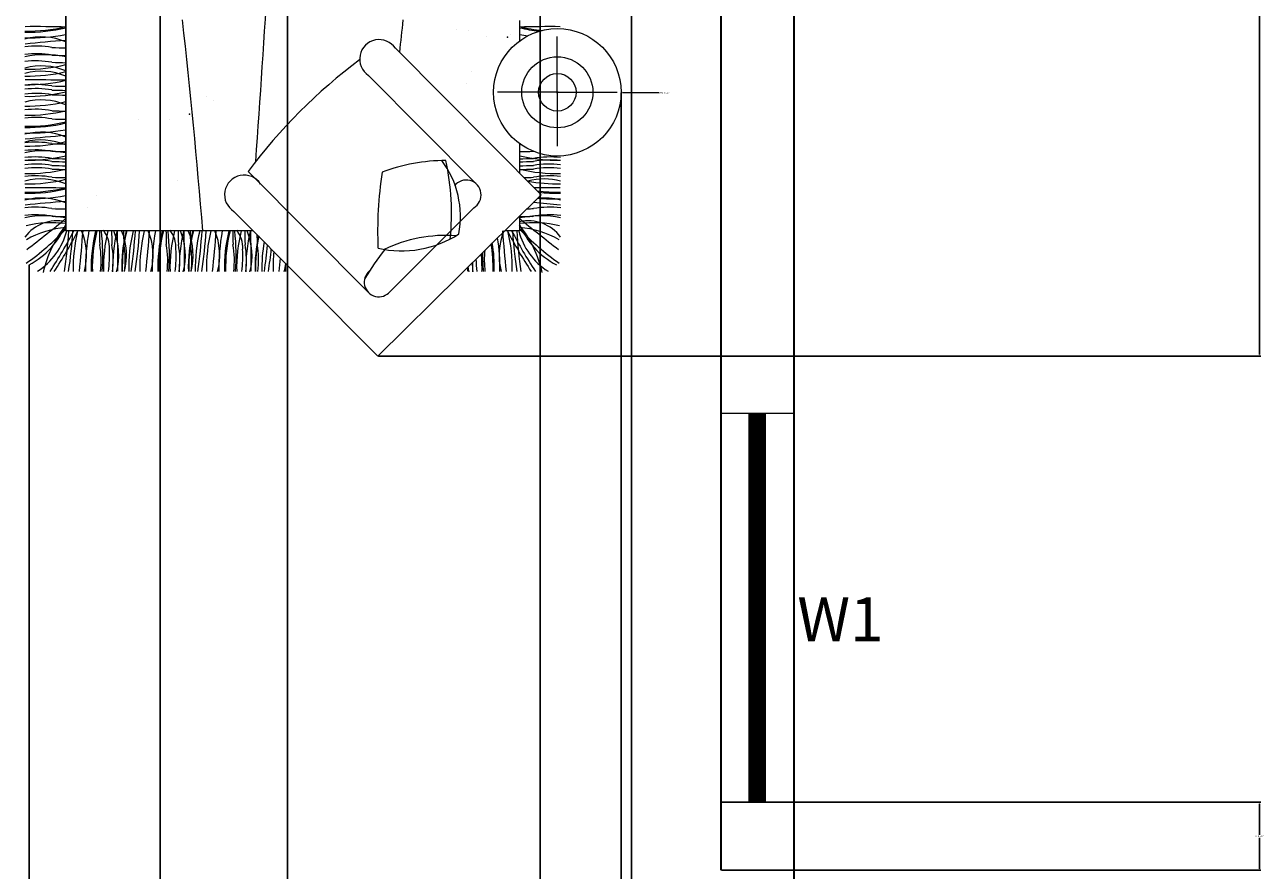
# Model space of a CAD drawing. Units: inches. Extents: x 318 to 927, y -1130 to 13.
# Tile 10 of 17: x 774 to 927, y -692 to -587. Entities that reach past the tile are written whole.
import ezdxf

# ---------------------------------------------------------------- set-up
doc = ezdxf.new("R2010")
doc.units = ezdxf.units.IN
doc.header["$MEASUREMENT"] = 0
for name, color, linetype, lineweight in [('A-ANNO-DIMS', 1, 'Continuous', 18), ('A-ANNO-IDEN', 1, 'Continuous', 13), ('A-FURN-RUGS', 50, 'Continuous', 9), ('A-GLAZ-PATT', 5, 'Continuous', 9), ('wall', 1, 'Continuous', 35), ('win', 5, 'Continuous', 18)]:
    doc.layers.add(name, color=color, linetype=linetype, lineweight=lineweight)
doc.layers.add('furniture', color=50, linetype='Continuous', lineweight=13, transparency=0.8)
doc.styles.get("Standard").update_dxf_attribs({"font": 'arial.ttf'})
doc.dimstyles.get("Standard").update_dxf_attribs({"dimtxt": 0.18, "dimasz": 0.18, "dimexe": 0.18, "dimexo": 0.0625, "dimgap": 0.09, "dimtad": 0, "dimtih": 1, "dimtoh": 1, "dimdec": 1, "dimzin": 0, "dimdsep": 46, "dimlunit": 4, "dimtxsty": 'Standard', "dimcen": 0.09, "dimadec": 0, "dimazin": 0, "dimtfac": 1, "dimtdec": 1, "dimtofl": 0, "dimtmove": 0, "dimatfit": 3, "dimfxl": 1, "dimtolj": 1, "dimtzin": 0, "dimarcsym": 0})

# ---------------------------------------------------------------- blocks, each defined once
blk = doc.blocks.new('WIN-48IN')
for p, q in [((0, 48), (9, 48)), ((3.5, 48), (3.5, 0)), ((5.5, 48), (5.5, 0)), ((0, 0), (9, 0))]:
    blk.add_line(p, q)
blk = doc.blocks.new('*D38')
at = {"layer": 'A-ANNO-DIMS', "color": 0, "lineweight": -2, "transparency": 16777216}
for p, q in [((817.59, -493.51), (926.57, -493.51)), ((926.39, -493.69), (926.39, -560.77)), ((926.39, -628.21), (926.39, -561.13)), ((817.59, -628.39), (926.57, -628.39))]:
    blk.add_line(p, q, dxfattribs=at)
at = {"layer": 'A-ANNO-DIMS', "color": 0, "transparency": 16777216}
for points in [[(926.36, -493.69), (926.42, -493.69), (926.39, -493.51)], [(926.36, -628.21), (926.42, -628.21), (926.39, -628.39)]]:
    blk.add_solid(points, dxfattribs=at)
at = {"layer": 'Defpoints', "color": 0, "transparency": 16777216}
for p in [(817.52, -493.51), (817.52, -628.39), (926.39, -628.39)]:
    blk.add_point(p, dxfattribs=at)
at = {"layer": 'A-ANNO-DIMS', "color": 0, "transparency": 16777216, "insert": (926.39, -560.95), "char_height": 0.18, "attachment_point": 5}
blk.add_mtext('\\A1;11\'-3"', dxfattribs=at)
blk = doc.blocks.new('*D39')
at = {"layer": 'A-ANNO-DIMS', "color": 0, "lineweight": -2, "transparency": 16777216}
for p, q in [((847.56, -595.87), (847.56, -1124.59)), ((774.46, -617.18), (774.46, -1124.59)), ((774.64, -1124.41), (810.68, -1124.41)), ((847.38, -1124.41), (811.34, -1124.41))]:
    blk.add_line(p, q, dxfattribs=at)
at = {"layer": 'A-ANNO-DIMS', "color": 0, "transparency": 16777216}
for points in [[(774.64, -1124.38), (774.64, -1124.44), (774.46, -1124.41)], [(847.38, -1124.38), (847.38, -1124.44), (847.56, -1124.41)]]:
    blk.add_solid(points, dxfattribs=at)
at = {"layer": 'Defpoints', "color": 0, "transparency": 16777216}
for p in [(847.56, -595.81), (774.46, -617.11), (847.56, -1124.41)]:
    blk.add_point(p, dxfattribs=at)
at = {"layer": 'A-ANNO-DIMS', "color": 0, "transparency": 16777216, "insert": (811.01, -1124.41), "char_height": 0.18, "attachment_point": 5}
blk.add_mtext('\\A1;6\'-1"', dxfattribs=at)
blk = doc.blocks.new('*D40')
at = {"layer": 'A-ANNO-DIMS', "color": 0, "lineweight": -2, "transparency": 16777216}
for p, q in [((790.65, -580.99), (790.65, -1124.59)), ((806.39, -580.99), (806.39, -1124.59)), ((790.83, -1124.41), (797.99, -1124.41)), ((806.21, -1124.41), (799.05, -1124.41))]:
    blk.add_line(p, q, dxfattribs=at)
at = {"layer": 'A-ANNO-DIMS', "color": 0, "transparency": 16777216}
for points in [[(790.83, -1124.38), (790.83, -1124.44), (790.65, -1124.41)], [(806.21, -1124.38), (806.21, -1124.44), (806.39, -1124.41)]]:
    blk.add_solid(points, dxfattribs=at)
at = {"layer": 'Defpoints', "color": 0, "transparency": 16777216}
for p in [(790.65, -580.93), (806.39, -580.93), (806.39, -1124.41)]:
    blk.add_point(p, dxfattribs=at)
at = {"layer": 'A-ANNO-DIMS', "color": 0, "transparency": 16777216, "insert": (798.52, -1124.41), "char_height": 0.18, "attachment_point": 5}
blk.add_mtext('\\A1;1\'-3 1/2"', dxfattribs=at)
blk = doc.blocks.new('*D53')
at = {"layer": 'A-ANNO-DIMS', "color": 0, "lineweight": -2, "transparency": 16777216}
for p, q in [((837.57, -839.31), (837.57, -25.23)), ((837.75, -25.41), (842.6, -25.41)), ((848.66, -25.41), (843.82, -25.41)), ((848.84, -838.59), (848.84, -25.23))]:
    blk.add_line(p, q, dxfattribs=at)
at = {"layer": 'A-ANNO-DIMS', "color": 0, "transparency": 16777216}
for points in [[(837.75, -25.38), (837.75, -25.44), (837.57, -25.41)], [(848.66, -25.38), (848.66, -25.44), (848.84, -25.41)]]:
    blk.add_solid(points, dxfattribs=at)
at = {"layer": 'Defpoints', "color": 0, "transparency": 16777216}
for p in [(848.84, -25.41), (837.57, -839.37), (848.84, -838.66)]:
    blk.add_point(p, dxfattribs=at)
at = {"layer": 'A-ANNO-DIMS', "color": 0, "transparency": 16777216, "insert": (843.21, -25.41), "char_height": 0.18, "attachment_point": 5}
blk.add_mtext('\\A1;0\'-11 1/2"', dxfattribs=at)
blk = doc.blocks.new('*D63')
at = {"layer": 'A-ANNO-DIMS', "color": 0, "lineweight": -2, "transparency": 16777216}
for p, q in [((859.96, -683.51), (926.57, -683.51)), ((926.39, -683.69), (926.39, -687.53)), ((926.39, -691.73), (926.39, -687.89)), ((859.96, -691.91), (926.57, -691.91))]:
    blk.add_line(p, q, dxfattribs=at)
at = {"layer": 'A-ANNO-DIMS', "color": 0, "transparency": 16777216}
for points in [[(926.36, -683.69), (926.42, -683.69), (926.39, -683.51)], [(926.36, -691.73), (926.42, -691.73), (926.39, -691.91)]]:
    blk.add_solid(points, dxfattribs=at)
at = {"layer": 'Defpoints', "color": 0, "transparency": 16777216}
for p in [(859.89, -683.51), (926.39, -683.51), (859.89, -691.91)]:
    blk.add_point(p, dxfattribs=at)
at = {"layer": 'A-ANNO-DIMS', "color": 0, "transparency": 16777216, "insert": (926.39, -687.71), "char_height": 0.18, "attachment_point": 5}
blk.add_mtext('\\A1;0\'-8 1/2"', dxfattribs=at)
blk = doc.blocks.new('*D72')
at = {"layer": 'A-ANNO-DIMS', "color": 0, "lineweight": -2, "transparency": 16777216}
for p, q in [((839.6, -595.81), (839.78, -595.81)), ((839.69, -595.9), (839.69, -595.72)), ((852.28, -595.87), (847.74, -595.85))]:
    blk.add_line(p, q, dxfattribs=at)
at = {"layer": 'A-ANNO-DIMS', "color": 0, "transparency": 16777216}
blk.add_solid([(847.74, -595.82), (847.74, -595.88), (847.56, -595.85)], dxfattribs=at)
at = {"layer": 'Defpoints', "color": 0, "transparency": 16777216}
for p in [(831.82, -595.77), (847.56, -595.85)]:
    blk.add_point(p, dxfattribs=at)
at = {"layer": 'A-ANNO-DIMS', "color": 0, "transparency": 16777216, "insert": (852.92, -595.87), "char_height": 0.18, "attachment_point": 5}
blk.add_mtext('\\A1;∅1\'-3 1/2"', dxfattribs=at)

msp = doc.modelspace()

# ---------------------------------------------------------------- hatches: boundary and pattern name
at = {"layer": 'A-GLAZ-PATT'}
h = msp.add_hatch(dxfattribs=at)
h.set_pattern_fill('ANSI31', color=256)
h.paths.add_polyline_path([(865.39, -312.52), (863.39, -312.52), (863.39, -348.52), (865.39, -348.52)])
h.paths.add_polyline_path([(865.39, -440.16), (863.39, -440.16), (863.39, -488.16), (865.39, -488.16)])
h.paths.add_polyline_path([(865.39, -635.51), (863.39, -635.51), (863.39, -683.51), (865.39, -683.51)])
h.paths.add_polyline_path([(865.39, -778.6), (863.39, -778.6), (863.39, -814.6), (865.39, -814.6)])
h.paths.add_polyline_path([(865.39, -834.21), (863.39, -834.21), (863.39, -870.21), (865.39, -870.21)])

# ---------------------------------------------------------------- linework, layer by layer
at = {"layer": 'A-FURN-RUGS'}
for p, q in [((779, -612.91), (779, -512.79)), ((779, -528.62), (779, -612.91)), ((835.03, -586.93), (835.03, -589.47)), ((827.23, -588.03), (827.23, -588.03)), ((828.75, -588.14), (828.75, -588.14)), ((833.86, -588.63), (833.86, -588.63)), ((830.93, -588.92), (830.93, -588.92)), ((829.14, -593.24), (829.14, -593.24)), ((828.42, -594.73), (828.42, -594.73)), ((796.39, -596.32), (796.39, -596.32)), ((796.39, -596.32), (796.39, -596.32)), ((797.21, -596.86), (797.21, -596.86)), ((797.21, -596.86), (797.21, -596.86)), ((788.03, -599.22), (788.03, -599.22)), ((791.76, -599.17), (791.76, -599.17)), ((794.51, -598.08), (794.51, -598.08)), ((835.03, -602.16), (835.03, -605.81)), ((792.76, -606.75), (792.76, -606.75)), ((782.8, -608.57), (782.8, -608.57)), ((777.71, -610.1), (777.71, -610.1)), ((777.71, -610.1), (777.71, -610.1)), ((777.71, -610.1), (777.71, -610.1)), ((781.73, -610.08), (781.73, -610.08)), ((836.32, -610.1), (836.32, -610.1)), ((836.32, -610.1), (836.32, -610.1)), ((836.32, -610.1), (836.32, -610.1)), ((777.42, -611.31), (777.42, -611.31)), ((777.42, -611.31), (777.42, -611.31)), ((777.42, -611.31), (777.42, -611.31)), ((835.03, -611.1), (835.03, -612.91)), ((836.61, -611.31), (836.61, -611.31)), ((836.61, -611.31), (836.61, -611.31)), ((836.61, -611.31), (836.61, -611.31)), ((802.13, -612.91), (779, -612.91)), ((835.03, -612.91), (833.2, -612.91)), ((786.52, -616.08), (786.52, -616.08)), ((786.56, -615.6), (786.56, -615.6)), ((794.75, -616.08), (794.75, -616.08)), ((794.79, -615.6), (794.79, -615.6)), ((802.98, -616.08), (802.98, -616.08)), ((803.02, -615.6), (803.02, -615.6))]:
    msp.add_line(p, q, dxfattribs=at)
for centre, radius, start, end in [((-3687.42, -292.9), 4500.67, 356.03178, 356.33069), ((-130.59, -689.06), 929.63, 4.69873, 6.31076), ((1744.62, -689.06), 929.63, 173.68924, 173.93736), ((774.4, -569.07), 19.18, 268.6331, 283.8573), ((774.4, -569.21), 19.18, 268.6331, 283.8573), ((774.37, -563.62), 25.47, 269.0195, 280.4039), ((775.11, -751.93), 164.23, 88.628, 90.3934), ((838.92, -751.93), 164.23, 89.6066, 91.372), ((839.63, -569.21), 19.18, 256.1427, 263.4467), ((839.63, -569.07), 19.18, 256.1427, 264.5854), ((839.66, -563.62), 25.47, 259.5961, 261.862), ((775.29, -601.49), 11.39, 79.9349, 96.8829), ((775.97, -596.84), 7.87, 67.3098, 104.8613), ((796.6, -812.63), 223.93, 94.5146, 95.8017), ((781.3, -463.32), 127.02, 268.1891, 268.9775), ((775.3, -602.44), 11.39, 79.9349, 96.8829), ((776.42, -603.93), 12.76, 78.4112, 101.2455), ((781.3, -464.27), 127.02, 268.1891, 268.9775), ((775.3, -603.32), 11.39, 79.9349, 96.8829), ((775.96, -601.08), 7.87, 67.3098, 104.8613), ((774.4, -574.63), 19.18, 268.6331, 283.8573), ((774.41, -573.77), 19.18, 268.6331, 283.8573), ((775.97, -600.42), 7.87, 67.3098, 104.8613), ((781.3, -465.15), 127.02, 268.1891, 268.9775), ((774.39, -575.7), 19.18, 268.6331, 283.8573), ((775.3, -606.24), 11.39, 79.9349, 96.8829), ((775.11, -758.51), 164.23, 88.628, 90.3934), ((774.39, -577.13), 19.18, 268.6331, 283.8573), ((775.3, -606.74), 11.39, 79.9349, 96.8829), ((775.31, -607.33), 11.39, 79.9349, 96.8829), ((781.3, -468.07), 127.02, 268.1891, 268.9775), ((781.3, -468.57), 127.02, 268.1891, 268.9775), ((781.31, -469.16), 127.02, 268.1891, 268.9775), ((775.95, -604.62), 7.87, 67.3098, 104.8613), ((774.39, -578.33), 19.18, 268.6331, 283.8573), ((775.3, -609.3), 11.39, 79.9349, 96.8829), ((774.4, -579.46), 19.18, 268.6331, 283.8573), ((775.3, -610.31), 11.39, 79.9349, 96.8829), ((774.4, -580.83), 19.18, 268.6331, 283.8573), ((781.31, -471.13), 127.02, 268.1891, 268.9775), ((781.31, -472.14), 127.02, 268.1891, 268.9775), ((774.4, -580.97), 19.18, 268.6331, 283.8573), ((774.37, -575.38), 25.47, 269.0195, 280.4039), ((775.97, -608.6), 7.87, 67.3098, 104.8613), ((775.95, -609.57), 7.87, 67.3098, 104.8613), ((774.39, -583.28), 19.18, 268.6331, 283.8573), ((775.29, -613.36), 11.39, 79.9349, 96.8829), ((796.6, -824.39), 223.93, 94.5146, 95.8017), ((781.3, -475.19), 127.02, 268.1891, 268.9775), ((832.73, -475.19), 127.02, 271.0225, 271.0606), ((838.08, -609.57), 7.87, 111.652, 112.6902), ((775.3, -614.32), 11.39, 79.9349, 96.8829), ((774.39, -585.02), 19.18, 268.6331, 283.8573), ((775.3, -615.19), 11.39, 79.9349, 96.8829), ((776.42, -615.8), 12.76, 78.4112, 101.2455), ((781.3, -476.14), 127.02, 268.1891, 268.9775), ((781.3, -477.02), 127.02, 268.1891, 268.9775), ((832.73, -476.14), 127.02, 271.0225, 271.8109), ((832.73, -477.02), 127.02, 271.0225, 271.8109), ((839.64, -585.02), 19.18, 256.1427, 271.3669), ((838.73, -615.19), 11.39, 83.1171, 100.0651), ((775.3, -615.56), 11.39, 79.9349, 96.8829), ((775.3, -616.06), 11.39, 79.9349, 96.8829), ((775.3, -616.52), 11.39, 79.9349, 96.8829), ((774.4, -586.67), 19.18, 268.6331, 283.8573), ((781.3, -477.39), 127.02, 268.1891, 268.9775), ((781.3, -477.89), 127.02, 268.1891, 268.9775), ((781.31, -478.34), 127.02, 268.1891, 268.9775), ((832.73, -477.39), 127.02, 271.0225, 271.8109), ((832.73, -477.89), 127.02, 271.0225, 271.8109), ((832.73, -478.34), 127.02, 271.0225, 271.8109), ((839.63, -586.67), 19.18, 256.1427, 271.3669), ((838.73, -615.56), 11.39, 83.1171, 100.0651), ((838.73, -616.06), 11.39, 83.1171, 100.0651), ((838.73, -616.52), 11.39, 83.1171, 100.0651), ((775.3, -617.52), 11.39, 79.9349, 96.8829), ((775.96, -614.39), 7.87, 67.3098, 104.8613), ((774.4, -587.94), 19.18, 268.6331, 283.8573), ((781.31, -479.35), 127.02, 268.1891, 268.9775), ((832.72, -479.35), 127.02, 271.2964, 271.8109), ((839.63, -587.94), 19.18, 259.2534, 271.3669), ((838.07, -614.39), 7.87, 75.1387, 104.8341), ((838.73, -617.52), 11.39, 83.1171, 100.0651), ((774.4, -588.97), 19.18, 268.6331, 283.8573), ((774.4, -589.11), 19.18, 268.6331, 283.8573), ((774.37, -583.52), 25.47, 269.0195, 280.4039), ((775.11, -771.83), 164.23, 88.628, 90.3934), ((838.92, -771.83), 164.23, 89.6066, 90.7304), ((839.63, -588.97), 19.18, 262.7707, 271.3669), ((839.63, -589.11), 19.18, 263.2584, 271.3669), ((775.29, -621.39), 11.39, 79.9349, 96.8829), ((775.97, -616.74), 7.87, 67.3098, 104.8613), ((796.6, -832.53), 223.93, 94.5146, 95.8017), ((817.43, -832.53), 223.93, 84.1983, 85.0575), ((838.74, -621.39), 11.39, 83.1171, 100.0651), ((838.07, -616.74), 7.87, 75.1387, 96.0041), ((839.66, -583.52), 25.47, 264.6488, 270.9805), ((775.3, -622.34), 11.39, 79.9349, 96.8829), ((776.42, -623.83), 12.76, 78.4112, 101.2455), ((777.91, -616.58), 4.9, 77.1946, 144.0943), ((679.49, -492.03), 155.39, 307.5441, 309.8432), ((781.3, -483.22), 127.02, 268.1891, 268.9775), ((781.3, -484.17), 127.02, 268.1891, 268.9775), ((934.54, -492.03), 155.39, 230.1568, 232.4559), ((832.73, -484.17), 127.02, 271.0225, 271.8109), ((836.12, -616.58), 4.9, 35.9057, 102.8054), ((837.61, -623.83), 12.76, 78.7545, 101.5888), ((832.73, -483.22), 127.02, 271.4616, 271.8109), ((838.74, -622.34), 11.39, 83.1171, 100.0651), ((777.27, -625.77), 13.84, 82.8509, 103.2785), ((754.54, -589.31), 33.84, 305.3153, 316.284), ((779.85, -623.99), 11.5, 94.2757, 119.865), ((770.01, -608.49), 9.7, 297.3033, 337.8819), ((771.07, -610.91), 8.28, 302.2712, 346.0065), ((790.74, -621.42), 14.92, 141.9231, 167.0477), ((729.8, -587.04), 56.46, 326.8219, 332.7331), ((730.31, -587.06), 56.46, 326.8219, 332.7331), ((724.61, -609.72), 54.84, 351.3771, 356.6356), ((725.12, -609.73), 54.84, 351.3771, 356.6356), ((799.08, -617.51), 19.18, 166.1427, 181.3669), ((557.89, -595.3), 223.93, 354.1983, 355.4854), ((773.68, -615.94), 7.87, 345.1387, 22.6902), ((806.9, -617.53), 25.47, 169.5961, 180.9805), ((801.3, -617.5), 19.18, 166.1427, 181.3669), ((801.45, -617.5), 19.18, 166.1427, 181.3669), ((910.14, -610.59), 127.02, 181.0225, 181.8109), ((757.66, -615.93), 25.91, 355.4936, 6.6298), ((802.82, -617.51), 19.18, 166.1427, 181.3669), ((780.95, -614.99), 3.43, 356.8256, 38.3436), ((911.64, -610.6), 127.02, 181.0225, 181.8109), ((803.95, -617.52), 19.18, 166.1427, 181.3669), ((777.66, -615.95), 7.87, 345.1387, 22.6902), ((621.19, -616.79), 164.23, 359.6066, 1.372), ((778.63, -615.94), 7.87, 345.1387, 22.6902), ((805.08, -617.5), 19.18, 166.1427, 181.3669), ((805.14, -617.51), 19.18, 166.1427, 181.3669), ((913.12, -610.59), 127.02, 181.0225, 181.8109), ((805.94, -617.5), 19.18, 166.1427, 181.3669), ((732.84, -609.72), 54.84, 351.3771, 356.6356), ((733.35, -609.73), 54.84, 351.3771, 356.6356), ((807.31, -617.51), 19.18, 166.1427, 181.3669), ((566.11, -595.3), 223.93, 354.1983, 355.4854), ((781.9, -615.94), 7.87, 345.1387, 22.6902), ((815.12, -617.53), 25.47, 169.5961, 180.9805), ((809.53, -617.5), 19.18, 166.1427, 181.3669), ((809.67, -617.5), 19.18, 166.1427, 181.3669), ((918.36, -610.59), 127.02, 181.0225, 181.8109), ((765.88, -615.93), 25.91, 355.4936, 6.6298), ((789.17, -614.99), 3.43, 356.8256, 38.3436), ((811.04, -617.51), 19.18, 166.1427, 181.3669), ((919.86, -610.6), 127.02, 181.0225, 181.8109), ((812.18, -617.52), 19.18, 166.1427, 181.3669), ((785.89, -615.95), 7.87, 345.1387, 22.6902), ((629.42, -616.79), 164.23, 359.6066, 1.372), ((786.85, -615.94), 7.87, 345.1387, 22.6902), ((813.3, -617.5), 19.18, 166.1427, 181.3669), ((813.37, -617.51), 19.18, 166.1427, 181.3669), ((921.35, -610.59), 127.02, 181.0225, 181.8109), ((814.16, -617.5), 19.18, 166.1427, 181.3669), ((741.07, -609.72), 54.84, 351.3771, 356.6356), ((741.58, -609.73), 54.84, 351.3771, 356.6356), ((815.54, -617.51), 19.18, 166.1427, 181.3669), ((574.34, -595.3), 223.93, 354.1983, 355.4854), ((790.13, -615.94), 7.87, 345.1387, 22.6902), ((823.36, -617.53), 25.47, 169.5961, 180.9805), ((817.76, -617.5), 19.18, 166.1427, 181.3669), ((817.9, -617.5), 19.18, 166.1427, 181.3669), ((926.6, -610.59), 127.02, 181.0225, 181.8109), ((774.12, -615.93), 25.91, 355.4936, 6.6298), ((819.27, -617.51), 19.18, 166.1427, 181.3669), ((797.41, -614.99), 3.43, 356.8256, 38.3436), ((928.09, -610.6), 127.02, 181.0225, 181.8109), ((820.41, -617.52), 19.18, 166.1427, 181.3669), ((794.12, -615.95), 7.87, 345.1387, 22.6902), ((637.65, -616.79), 164.23, 359.6066, 1.372), ((840.36, -615.94), 7.87, 157.3098, 194.8613), ((1056.15, -595.3), 223.93, 184.5146, 185.8017), ((883.72, -587.06), 56.46, 207.2669, 213.1781), ((814.95, -617.51), 19.18, 358.6331, 13.8573), ((884.23, -587.04), 56.46, 207.2669, 213.1781), ((888.91, -609.73), 54.84, 183.3644, 188.6229), ((889.42, -609.72), 54.84, 183.3644, 188.6229), ((842.96, -610.91), 8.28, 193.9935, 237.7288), ((836.76, -625.77), 13.84, 76.7215, 97.1491), ((844.02, -608.49), 9.7, 202.1181, 242.6967), ((823.29, -621.42), 14.92, 12.9523, 38.0769), ((834.18, -623.99), 11.5, 60.135, 85.7243), ((859.49, -589.31), 33.84, 223.716, 234.6847), ((771.97, -616.6), 11.39, 353.1171, 10.0651), ((773.46, -616.6), 11.39, 353.1171, 10.0651), ((774.95, -616.59), 11.39, 353.1171, 10.0651), ((780.19, -616.6), 11.39, 353.1171, 10.0651), ((781.69, -616.6), 11.39, 353.1171, 10.0651), ((783.17, -616.59), 11.39, 353.1171, 10.0651), ((788.42, -616.6), 11.39, 353.1171, 10.0651), ((789.92, -616.6), 11.39, 353.1171, 10.0651), ((821.54, -617.5), 19.18, 168.0993, 181.3669), ((821.6, -617.51), 19.18, 168.2362, 181.3669), ((929.58, -610.59), 127.02, 181.2535, 181.8109), ((791.41, -616.59), 11.39, 353.1171, 10.0651), ((822.39, -617.5), 19.18, 170.3159, 181.3669), ((749.29, -609.72), 54.84, 351.3771, 354.7986), ((812.58, -617.5), 19.18, 358.6331, 8.8561), ((812.73, -617.5), 19.18, 358.6331, 9.2236), ((807.13, -617.53), 25.47, 359.0195, 8.4847), ((766.64, -615.97), 17.75, 353.5587, 2.5565), ((774.87, -615.97), 17.75, 353.5587, 2.5565), ((783.1, -615.97), 17.75, 353.5587, 2.5565), ((749.8, -609.73), 54.84, 351.3771, 354.3194), ((823.76, -617.51), 19.18, 173.9229, 181.3669), ((811.21, -617.51), 19.18, 358.6331, 5.2422), ((856.37, -615.93), 25.91, 179.2987, 184.5064), ((842.06, -616.6), 11.39, 173.6069, 186.8829), ((582.57, -595.3), 223.93, 354.1983, 354.6171), ((798.36, -615.94), 7.87, 345.1387, 352.5478), ((831.58, -617.53), 25.47, 178.619, 180.9805), ((992.84, -616.79), 164.23, 180.2284, 180.3934), ((836.37, -615.95), 7.87, 190.6792, 194.8613), ((840.57, -616.6), 11.39, 181.3666, 186.8829), ((810.08, -617.52), 19.18, 358.6331, 2.1135), ((847.39, -615.97), 17.75, 181.4332, 186.4413)]:
    msp.add_arc(centre, radius, start, end, dxfattribs=at)
for p in [(833.52, -588.98), (794.27, -598.51)]:
    msp.add_point(p, dxfattribs=at)
at = {"layer": 'furniture'}
for p, q in [((839.69, -595.81), (839.69, -588.92)), ((837.69, -608.48), (819.69, -590.37)), ((829.74, -607.2), (816.35, -593.71)), ((839.69, -595.81), (832.32, -595.81)), ((839.69, -595.81), (839.69, -602.45)), ((839.69, -595.81), (847.06, -595.81)), ((801.51, -605.6), (816.37, -620.54)), ((837.69, -608.48), (817.52, -628.39)), ((829.38, -610.08), (819.03, -620.42)), ((829.38, -610.08), (827.72, -611.74)), ((817.52, -628.39), (799.75, -610.52)), ((824.8, -614.65), (819.03, -620.42))]:
    msp.add_line(p, q, dxfattribs=at)
for radius in [7.87, 4.39, 2.32]:
    msp.add_circle((839.69, -595.81), radius, dxfattribs=at)
for centre, radius, start, end in [((817.69, -591.71), 2.41, 33.6335, 236.3665), ((855.25, -645.52), 66.95, 126.6613, 143.3951), ((826.05, -626.98), 22.75, 90.3068, 110.5663), ((816.13, -611.18), 11.6, 349.4501, 36.7699), ((795.91, -610.76), 30.72, 354.0815, 12.2768), ((801.02, -608.46), 2.42, 33.0924, 238.5307), ((866.17, -613.01), 48.67, 171.3371, 182.4176), ((828.44, -608.49), 1.84, 300.4819, 142.3252), ((820.47, -602.4), 13, 257.0126, 302.9429), ((825.92, -631.08), 17.59, 85.9005, 115.6513), ((846.21, -637.09), 35.39, 141.8457, 148.9133), ((817.65, -619.26), 1.81, 130.1092, 319.8908)]:
    msp.add_arc(centre, radius, start, end, dxfattribs=at)
at = {"layer": 'wall'}
for p, q in [((868.89, -82.91), (868.89, -1042.91)), ((859.89, -433.91), (859.89, -691.91))]:
    msp.add_line(p, q, dxfattribs=at)

# ---------------------------------------------------------------- block references
at = {"layer": 'win', "rotation": 180}
msp.add_blockref('WIN-48IN', (868.89, -635.51), dxfattribs=at)

# ---------------------------------------------------------------- texts
at = {"layer": 'A-ANNO-IDEN'}
msp.add_text('W1', height=5.444, dxfattribs=at).set_placement((869.32, -663.63))

# ---------------------------------------------------------------- dimensions: what is measured, and where the dimension line sits
at = {"layer": 'A-ANNO-DIMS'}
for base, p1, p2, picture, middle in [((848.84, -25.41), (837.57, -839.37), (848.84, -838.66), '*D53', (843.21, -25.41)), ((806.39, -1124.41), (790.65, -580.93), (806.39, -580.93), '*D40', (798.52, -1124.41)), ((847.56, -1124.41), (774.46, -617.11), (847.56, -595.81), '*D39', (811.01, -1124.41))]:
    dim = msp.add_linear_dim(base=base, p1=p1, p2=p2, dimstyle='Standard', override={"dimdec": 1, "dimlfac": 1, "dimrnd": 0, "dimzin": 1, "dimdsep": 46, "dimlunit": 4, "dimfrac": 2}, dxfattribs=at)
    dim.commit()
    dim.dimension.update_dxf_attribs({"geometry": picture, "text_midpoint": middle})
for base, p1, p2, picture, middle in [((926.39, -628.39), (817.52, -493.51), (817.52, -628.39), '*D38', (926.39, -560.95)), ((926.39, -683.51), (859.89, -691.91), (859.89, -683.51), '*D63', (926.39, -687.71))]:
    dim = msp.add_linear_dim(base=base, p1=p1, p2=p2, angle=90, dimstyle='Standard', override={"dimdec": 1, "dimlfac": 1, "dimrnd": 0, "dimzin": 1, "dimdsep": 46, "dimlunit": 4, "dimfrac": 2}, dxfattribs=at)
    dim.commit()
    dim.dimension.update_dxf_attribs({"geometry": picture, "text_midpoint": middle})
dim = msp.add_diameter_dim_2p(p1=(831.82, -595.77), p2=(847.56, -595.85), dimstyle='Standard', override={"dimdec": 1, "dimlfac": 1, "dimrnd": 0, "dimzin": 1, "dimdsep": 46, "dimlunit": 4, "dimfrac": 2}, dxfattribs=at)
dim.commit()
dim.dimension.update_dxf_attribs({"geometry": '*D72', "text_midpoint": (852.28, -595.87), "dimtype": 163})

doc.saveas('drawing.dxf')
